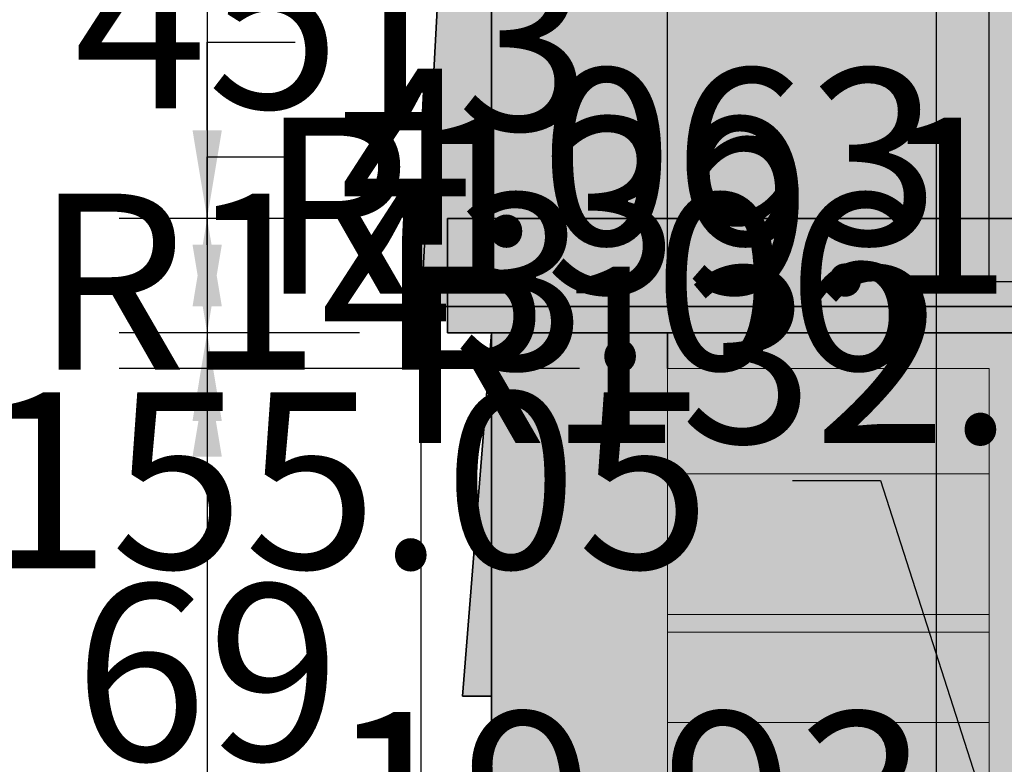
# Model space of a CAD drawing. Units: millimetres. Extents: x 130 to 1021, y 147 to 699.
# Tile 17 of 40: x 254 to 366, y 525 to 610. Entities that reach past the tile are written whole.
import ezdxf

# ---------------------------------------------------------------- set-up
doc = ezdxf.new("R2010")
doc.units = ezdxf.units.MM
doc.header["$MEASUREMENT"] = 0
for name, color, linetype, lineweight in [('A-ANNO-DIMS', 2, 'Continuous', 18), ('A-ELEV', 7, 'Continuous', 35), ('A-ELEV-PATT', 9, 'Continuous', 13), ('A-GLAZ', 4, 'Continuous', 18)]:
    doc.layers.add(name, color=color, linetype=linetype, lineweight=lineweight)
doc.styles.get("Standard").update_dxf_attribs({"font": 'arial.ttf'})
doc.dimstyles.get("Standard").update_dxf_attribs({"dimtxt": 20, "dimasz": 10, "dimexe": 10, "dimexo": 10, "dimgap": 5, "dimtad": 0, "dimtih": 1, "dimtoh": 1, "dimdec": 0, "dimzin": 0, "dimdsep": 46, "dimtxsty": 'Standard', "dimcen": 5, "dimadec": 0, "dimazin": 0, "dimtfac": 1, "dimtdec": 0, "dimtofl": 0, "dimtmove": 0, "dimatfit": 3, "dimfxl": 1, "dimtolj": 1, "dimtzin": 0, "dimarcsym": 0})

# ---------------------------------------------------------------- blocks, each defined once
blk = doc.blocks.new('*D11')
at = {"layer": 'A-ANNO-DIMS', "color": 0, "lineweight": -2, "transparency": 16777216}
for p, q in [((737.37, 648.7), (737.37, 149.74)), ((299.37, 566.95), (299.37, 149.74)), ((309.37, 159.74), (490.86, 159.74)), ((727.37, 159.74), (545.89, 159.74))]:
    blk.add_line(p, q, dxfattribs=at)
at = {"layer": 'A-ANNO-DIMS', "color": 0, "transparency": 16777216}
for points in [[(309.37, 161.41), (309.37, 158.07), (299.37, 159.74)], [(727.37, 161.41), (727.37, 158.07), (737.37, 159.74)]]:
    blk.add_solid(points, dxfattribs=at)
at = {"layer": 'Defpoints', "color": 0, "transparency": 16777216}
for p in [(737.37, 658.7), (299.37, 576.95), (737.37, 159.74)]:
    blk.add_point(p, dxfattribs=at)
at = {"layer": 'A-ANNO-DIMS', "color": 0, "transparency": 16777216, "insert": (518.37, 159.74), "char_height": 20, "attachment_point": 5}
blk.add_mtext('\\A1;438', dxfattribs=at)
blk = doc.blocks.new('*D12')
at = {"layer": 'A-ANNO-DIMS', "color": 0, "lineweight": -2, "transparency": 16777216}
for p, q in [((477.37, 661.95), (265.07, 661.95)), ((275.07, 651.95), (275.07, 438.2)), ((275.07, 194.04), (275.07, 407.78)), ((357.16, 184.04), (265.07, 184.04))]:
    blk.add_line(p, q, dxfattribs=at)
at = {"layer": 'A-ANNO-DIMS', "color": 0, "transparency": 16777216}
for points in [[(273.41, 651.95), (276.74, 651.95), (275.07, 661.95)], [(273.41, 194.04), (276.74, 194.04), (275.07, 184.04)]]:
    blk.add_solid(points, dxfattribs=at)
at = {"layer": 'Defpoints', "color": 0, "transparency": 16777216}
for p in [(275.07, 661.95), (487.37, 661.95), (367.16, 184.04)]:
    blk.add_point(p, dxfattribs=at)
at = {"layer": 'A-ANNO-DIMS', "color": 0, "transparency": 16777216, "insert": (275.07, 422.99), "char_height": 20, "attachment_point": 5}
blk.add_mtext('\\A1;477.9', dxfattribs=at)
blk = doc.blocks.new('*D14')
at = {"layer": 'A-ANNO-DIMS', "color": 0, "lineweight": -2, "transparency": 16777216}
for p, q in [((307.37, 641.95), (307.37, 696.25)), ((327.37, 579.88), (327.37, 696.25)), ((297.37, 686.25), (287.37, 686.25)), ((337.37, 686.25), (347.37, 686.25))]:
    blk.add_line(p, q, dxfattribs=at)
at = {"layer": 'A-ANNO-DIMS', "color": 0, "transparency": 16777216}
for points in [[(297.37, 687.91), (297.37, 684.58), (307.37, 686.25)], [(337.37, 687.91), (337.37, 684.58), (327.37, 686.25)]]:
    blk.add_solid(points, dxfattribs=at)
at = {"layer": 'Defpoints', "color": 0, "transparency": 16777216}
for p in [(327.37, 686.25), (307.37, 631.95), (327.37, 569.88)]:
    blk.add_point(p, dxfattribs=at)
at = {"layer": 'A-ANNO-DIMS', "color": 0, "transparency": 16777216, "insert": (366.83, 686.25), "char_height": 20, "attachment_point": 5}
blk.add_mtext('\\A1;20', dxfattribs=at)
blk = doc.blocks.new('*D15')
at = {"layer": 'A-ANNO-DIMS', "color": 0, "lineweight": -2, "transparency": 16777216}
for p, q in [((327.37, 579.88), (327.37, 696.25)), ((357.94, 411.95), (357.94, 696.25)), ((337.37, 686.25), (347.94, 686.25)), ((357.94, 686.25), (367.94, 686.25))]:
    blk.add_line(p, q, dxfattribs=at)
at = {"layer": 'A-ANNO-DIMS', "color": 0, "transparency": 16777216}
for points in [[(337.37, 687.91), (337.37, 684.58), (327.37, 686.25)], [(347.94, 687.91), (347.94, 684.58), (357.94, 686.25)]]:
    blk.add_solid(points, dxfattribs=at)
at = {"layer": 'Defpoints', "color": 0, "transparency": 16777216}
for p in [(357.94, 686.25), (327.37, 569.88), (357.94, 401.95)]:
    blk.add_point(p, dxfattribs=at)
at = {"layer": 'A-ANNO-DIMS', "color": 0, "transparency": 16777216, "insert": (406.68, 686.25), "char_height": 20, "attachment_point": 5}
blk.add_mtext('\\A1;30.57', dxfattribs=at)
blk = doc.blocks.new('*D16')
at = {"layer": 'A-ANNO-DIMS', "color": 0, "lineweight": -2, "transparency": 16777216}
for p, q in [((357.94, 411.95), (357.94, 696.25)), ((363.92, 579.88), (363.92, 696.25)), ((347.94, 686.25), (337.94, 686.25)), ((373.92, 686.25), (383.92, 686.25))]:
    blk.add_line(p, q, dxfattribs=at)
at = {"layer": 'A-ANNO-DIMS', "color": 0, "transparency": 16777216}
for points in [[(347.94, 687.91), (347.94, 684.58), (357.94, 686.25)], [(373.92, 687.91), (373.92, 684.58), (363.92, 686.25)]]:
    blk.add_solid(points, dxfattribs=at)
at = {"layer": 'Defpoints', "color": 0, "transparency": 16777216}
for p in [(363.92, 686.25), (363.92, 569.88), (357.94, 401.95)]:
    blk.add_point(p, dxfattribs=at)
at = {"layer": 'A-ANNO-DIMS', "color": 0, "transparency": 16777216, "insert": (420.74, 686.25), "char_height": 20, "attachment_point": 5}
blk.add_mtext('\\A1;5.981', dxfattribs=at)
blk = doc.blocks.new('*D17')
at = {"layer": 'A-ANNO-DIMS', "color": 0, "lineweight": -2, "transparency": 16777216}
for p, q in [((363.92, 579.88), (363.92, 696.25)), ((375.85, 490.22), (375.85, 696.25)), ((353.92, 686.25), (343.92, 686.25)), ((385.85, 686.25), (395.85, 686.25))]:
    blk.add_line(p, q, dxfattribs=at)
at = {"layer": 'A-ANNO-DIMS', "color": 0, "transparency": 16777216}
for points in [[(353.92, 687.91), (353.92, 684.58), (363.92, 686.25)], [(385.85, 687.91), (385.85, 684.58), (375.85, 686.25)]]:
    blk.add_solid(points, dxfattribs=at)
at = {"layer": 'Defpoints', "color": 0, "transparency": 16777216}
for p in [(375.85, 686.25), (363.92, 569.88), (375.85, 480.22)]:
    blk.add_point(p, dxfattribs=at)
at = {"layer": 'A-ANNO-DIMS', "color": 0, "transparency": 16777216, "insert": (441.44, 686.25), "char_height": 20, "attachment_point": 5}
blk.add_mtext('\\A1;11.928', dxfattribs=at)
blk = doc.blocks.new('*D18')
at = {"layer": 'A-ANNO-DIMS', "color": 0, "lineweight": -2, "transparency": 16777216}
for p, q in [((375.85, 490.22), (375.85, 696.25)), ((382.37, 388.95), (382.37, 696.25)), ((365.85, 686.25), (355.85, 686.25)), ((392.37, 686.25), (402.37, 686.25))]:
    blk.add_line(p, q, dxfattribs=at)
at = {"layer": 'A-ANNO-DIMS', "color": 0, "transparency": 16777216}
for points in [[(365.85, 687.91), (365.85, 684.58), (375.85, 686.25)], [(392.37, 687.91), (392.37, 684.58), (382.37, 686.25)]]:
    blk.add_solid(points, dxfattribs=at)
at = {"layer": 'Defpoints', "color": 0, "transparency": 16777216}
for p in [(382.37, 686.25), (375.85, 480.22), (382.37, 378.95)]:
    blk.add_point(p, dxfattribs=at)
at = {"layer": 'A-ANNO-DIMS', "color": 0, "transparency": 16777216, "insert": (441.13, 686.25), "char_height": 20, "attachment_point": 5}
blk.add_mtext('\\A1;6.524', dxfattribs=at)
blk = doc.blocks.new('*D43')
at = {"layer": 'A-ANNO-DIMS', "color": 0, "lineweight": -2, "transparency": 16777216}
for p, q in [((275.07, 510.88), (275.07, 520.88)), ((275.07, 520.88), (285.07, 520.88)), ((404.65, 500.88), (265.07, 500.88)), ((317.37, 480.95), (265.07, 480.95)), ((275.07, 470.95), (275.07, 460.95))]:
    blk.add_line(p, q, dxfattribs=at)
at = {"layer": 'A-ANNO-DIMS', "color": 0, "transparency": 16777216}
for points in [[(273.41, 510.88), (276.74, 510.88), (275.07, 500.88)], [(273.41, 470.95), (276.74, 470.95), (275.07, 480.95)]]:
    blk.add_solid(points, dxfattribs=at)
at = {"layer": 'Defpoints', "color": 0, "transparency": 16777216}
for p in [(275.07, 500.88), (414.65, 500.88), (327.37, 480.95)]:
    blk.add_point(p, dxfattribs=at)
at = {"layer": 'A-ANNO-DIMS', "color": 0, "transparency": 16777216, "insert": (322.88, 520.88), "char_height": 20, "attachment_point": 5}
blk.add_mtext('\\A1;19.93', dxfattribs=at)
blk = doc.blocks.new('*D44')
at = {"layer": 'A-ANNO-DIMS', "color": 0, "lineweight": -2, "transparency": 16777216}
for p, q in [((317.37, 569.88), (265.07, 569.88)), ((275.07, 559.88), (275.07, 550.59)), ((275.07, 510.88), (275.07, 520.17)), ((404.65, 500.88), (265.07, 500.88))]:
    blk.add_line(p, q, dxfattribs=at)
at = {"layer": 'A-ANNO-DIMS', "color": 0, "transparency": 16777216}
for points in [[(273.41, 559.88), (276.74, 559.88), (275.07, 569.88)], [(273.41, 510.88), (276.74, 510.88), (275.07, 500.88)]]:
    blk.add_solid(points, dxfattribs=at)
at = {"layer": 'Defpoints', "color": 0, "transparency": 16777216}
for p in [(275.07, 569.88), (327.37, 569.88), (414.65, 500.88)]:
    blk.add_point(p, dxfattribs=at)
at = {"layer": 'A-ANNO-DIMS', "color": 0, "transparency": 16777216, "insert": (275.07, 535.38), "char_height": 20, "attachment_point": 5}
blk.add_mtext('\\A1;69', dxfattribs=at)
blk = doc.blocks.new('*D45')
at = {"layer": 'A-ANNO-DIMS', "color": 0, "lineweight": -2, "transparency": 16777216}
for p, q in [((275.07, 583.95), (275.07, 593.95)), ((275.07, 593.95), (285.07, 593.95)), ((292.37, 573.95), (265.07, 573.95)), ((317.37, 569.88), (265.07, 569.88)), ((275.07, 559.88), (275.07, 549.88))]:
    blk.add_line(p, q, dxfattribs=at)
at = {"layer": 'A-ANNO-DIMS', "color": 0, "transparency": 16777216}
for points in [[(273.41, 583.95), (276.74, 583.95), (275.07, 573.95)], [(273.41, 559.88), (276.74, 559.88), (275.07, 569.88)]]:
    blk.add_solid(points, dxfattribs=at)
at = {"layer": 'Defpoints', "color": 0, "transparency": 16777216}
for p in [(275.07, 573.95), (302.37, 573.95), (327.37, 569.88)]:
    blk.add_point(p, dxfattribs=at)
at = {"layer": 'A-ANNO-DIMS', "color": 0, "transparency": 16777216, "insert": (324.22, 593.95), "char_height": 20, "attachment_point": 5}
blk.add_mtext('\\A1;4.063', dxfattribs=at)
blk = doc.blocks.new('*D46')
at = {"layer": 'A-ANNO-DIMS', "color": 0, "lineweight": -2, "transparency": 16777216}
for p, q in [((275.07, 596.95), (275.07, 606.95)), ((275.07, 606.95), (285.07, 606.95)), ((292.37, 586.95), (265.07, 586.95)), ((292.37, 573.95), (265.07, 573.95)), ((275.07, 563.95), (275.07, 553.95))]:
    blk.add_line(p, q, dxfattribs=at)
at = {"layer": 'A-ANNO-DIMS', "color": 0, "transparency": 16777216}
for points in [[(273.41, 596.95), (276.74, 596.95), (275.07, 586.95)], [(273.41, 563.95), (276.74, 563.95), (275.07, 573.95)]]:
    blk.add_solid(points, dxfattribs=at)
at = {"layer": 'Defpoints', "color": 0, "transparency": 16777216}
for p in [(275.07, 586.95), (302.37, 586.95), (302.37, 573.95)]:
    blk.add_point(p, dxfattribs=at)
at = {"layer": 'A-ANNO-DIMS', "color": 0, "transparency": 16777216, "insert": (303.46, 606.95), "char_height": 20, "attachment_point": 5}
blk.add_mtext('\\A1;13', dxfattribs=at)
blk = doc.blocks.new('*D47')
at = {"layer": 'A-ANNO-DIMS', "color": 0, "lineweight": -2, "transparency": 16777216}
for p, q in [((275.07, 641.95), (275.07, 651.95)), ((292.37, 631.95), (265.07, 631.95)), ((292.37, 586.95), (265.07, 586.95)), ((275.07, 576.95), (275.07, 566.95))]:
    blk.add_line(p, q, dxfattribs=at)
at = {"layer": 'A-ANNO-DIMS', "color": 0, "transparency": 16777216}
for points in [[(273.41, 641.95), (276.74, 641.95), (275.07, 631.95)], [(273.41, 576.95), (276.74, 576.95), (275.07, 586.95)]]:
    blk.add_solid(points, dxfattribs=at)
at = {"layer": 'Defpoints', "color": 0, "transparency": 16777216}
for p in [(275.07, 631.95), (302.37, 631.95), (302.37, 586.95)]:
    blk.add_point(p, dxfattribs=at)
at = {"layer": 'A-ANNO-DIMS', "color": 0, "transparency": 16777216, "insert": (275.07, 609.45), "char_height": 20, "attachment_point": 5}
blk.add_mtext('\\A1;45', dxfattribs=at)
blk = doc.blocks.new('*D66')
at = {"layer": 'A-ANNO-DIMS', "color": 0, "lineweight": -2, "transparency": 16777216}
for p, q in [((341.58, 557.19), (351.58, 557.19)), ((351.58, 557.19), (376.95, 478.14)), ((427.37, 315.98), (427.37, 325.98)), ((422.37, 320.98), (432.37, 320.98))]:
    blk.add_line(p, q, dxfattribs=at)
at = {"layer": 'A-ANNO-DIMS', "color": 0, "transparency": 16777216}
blk.add_solid([(378.53, 478.64), (375.36, 477.63), (380, 468.61)], dxfattribs=at)
at = {"layer": 'Defpoints', "color": 0, "transparency": 16777216}
for p in [(380, 468.61), (427.37, 320.98)]:
    blk.add_point(p, dxfattribs=at)
at = {"layer": 'A-ANNO-DIMS', "color": 0, "transparency": 16777216, "insert": (263.53, 557.19), "char_height": 20, "attachment_point": 5}
blk.add_mtext('\\A1;4X R155.05', dxfattribs=at)
blk = doc.blocks.new('*D68')
at = {"layer": 'A-ANNO-DIMS', "color": 0, "lineweight": -2, "transparency": 16777216}
for p, q in [((361.84, 579.76), (371.84, 579.76)), ((371.84, 579.76), (392.17, 506.69)), ((433.19, 354.23), (433.19, 364.23)), ((428.19, 359.23), (438.19, 359.23))]:
    blk.add_line(p, q, dxfattribs=at)
at = {"layer": 'A-ANNO-DIMS', "color": 0, "transparency": 16777216}
blk.add_solid([(393.77, 507.14), (390.56, 506.25), (394.85, 497.06)], dxfattribs=at)
at = {"layer": 'Defpoints', "color": 0, "transparency": 16777216}
for p in [(394.85, 497.06), (433.19, 359.23)]:
    blk.add_point(p, dxfattribs=at)
at = {"layer": 'A-ANNO-DIMS', "color": 0, "transparency": 16777216, "insert": (305.76, 579.76), "char_height": 20, "attachment_point": 5}
blk.add_mtext('\\A1;R143.06', dxfattribs=at)
blk = doc.blocks.new('*D70')
at = {"layer": 'A-ANNO-DIMS', "color": 0, "lineweight": -2, "transparency": 16777216}
for p, q in [((370.14, 588.4), (380.14, 588.4)), ((380.14, 588.4), (397.47, 517.01)), ((432.65, 367.11), (432.65, 377.11)), ((427.65, 372.11), (437.65, 372.11))]:
    blk.add_line(p, q, dxfattribs=at)
at = {"layer": 'A-ANNO-DIMS', "color": 0, "transparency": 16777216}
blk.add_solid([(399.09, 517.4), (395.85, 516.62), (399.83, 507.29)], dxfattribs=at)
at = {"layer": 'Defpoints', "color": 0, "transparency": 16777216}
for p in [(399.83, 507.29), (432.65, 372.11)]:
    blk.add_point(p, dxfattribs=at)
at = {"layer": 'A-ANNO-DIMS', "color": 0, "transparency": 16777216, "insert": (323.76, 588.4), "char_height": 20, "attachment_point": 5}
blk.add_mtext('\\A1;R139.1', dxfattribs=at)
blk = doc.blocks.new('*D73')
at = {"layer": 'A-ANNO-DIMS', "color": 0, "lineweight": -2, "transparency": 16777216}
for p, q in [((402.68, 571.45), (412.68, 571.45)), ((412.68, 571.45), (419.05, 502.17)), ((432.11, 355.14), (432.11, 365.14)), ((427.11, 360.14), (437.11, 360.14))]:
    blk.add_line(p, q, dxfattribs=at)
at = {"layer": 'A-ANNO-DIMS', "color": 0, "transparency": 16777216}
blk.add_solid([(420.71, 502.32), (417.39, 502.01), (419.97, 492.21)], dxfattribs=at)
at = {"layer": 'Defpoints', "color": 0, "transparency": 16777216}
for p in [(419.97, 492.21), (432.11, 360.14)]:
    blk.add_point(p, dxfattribs=at)
at = {"layer": 'A-ANNO-DIMS', "color": 0, "transparency": 16777216, "insert": (346.7, 571.45), "char_height": 20, "attachment_point": 5}
blk.add_mtext('\\A1;R132.62', dxfattribs=at)

msp = doc.modelspace()

# ---------------------------------------------------------------- hatches: boundary and pattern name
at = {"layer": 'A-ELEV-PATT'}
h = msp.add_hatch(color=256, dxfattribs=at)
h.dxf.hatch_style = 1
h.paths.add_polyline_path([(737.3738, 658.6988, 0.01359606), (632.4019, 661.9473), (607.3738, 661.9473), (487.3738, 661.9473), (487.3738, 649.9473), (607.3738, 649.9473), (632.3794, 649.9473, -0.01368411), (737.3738, 646.6784)])
h.paths.add_polyline_path([(732.3738, 643.9599, 0.01305286), (632.3738, 646.9473), (607.3738, 646.9473), (487.3738, 646.9473), (487.3738, 596.9473), (632.3738, 596.9473, -0.01305286), (732.3738, 593.9599)])
h.paths.add_polyline_path([(737.3738, 593.6732, 0.01370629), (632.3738, 596.9473), (487.3738, 596.9473), (487.3738, 586.9473), (632.355, 586.9473, -0.01378075), (737.3738, 583.6559)])
h.paths.add_polyline_path([(447.3738, 646.9473), (307.3738, 646.9473), (302.3738, 646.9473), (302.3738, 634.9473), (447.3738, 634.9473)])
h.paths.add_polyline_path([(447.3738, 631.9473), (307.3738, 631.9473), (307.3738, 586.9473), (447.3738, 586.9473)])
h.paths.add_polyline_path([(447.3738, 586.9473), (307.3738, 586.9473), (302.3738, 586.9473), (302.3738, 576.9473), (447.3738, 576.9473)])
h.paths.add_polyline_path([(447.3738, 573.9473), (367.3738, 573.9473), (367.3738, 539.9473), (447.3738, 539.9473)])
h.paths.add_polyline_path([(447.3738, 537.9473), (367.3738, 537.9473), (367.3738, 507.9473), (400.392, 507.4253, -0.00172798), (401.3281, 507.6451, -0.52200255), (425.6117, 511.0391, -0.03918489), (447.3738, 510.4359), (447.3738, 510.7883)])
h.paths.add_polyline_path([(394.7238, 505.9473), (367.3738, 505.9473), (367.3738, 476.9473, -0.0146512), (375.8501, 480.2159), (376.1506, 499.2266, -0.03554194)])
h.paths.add_polyline_path([(632.3738, 583.9473), (552.3738, 583.9473), (552.3738, 550.9473), (632.3738, 550.9473)])
h.paths.add_polyline_path([(632.3738, 548.9473), (552.3738, 548.9473), (552.3738, 515.9473), (632.3738, 515.9473)])
h.paths.add_polyline_path([(632.3738, 513.9473), (552.3738, 513.9473), (552.3738, 476.9473), (632.3738, 476.9473)])
h.paths.add_polyline_path([(737.3738, 473.6903, 0.01363261), (632.3926, 476.9473), (552.3738, 476.9473), (487.3738, 476.9473), (487.3738, 466.9473), (632.3738, 466.9473, -0.01370629), (737.3738, 463.6732)])
h.paths.add_polyline_path([(732.3738, 460.9552, 0.01307409), (632.3681, 463.9473), (487.3738, 463.9473), (487.3738, 407.735, -0.00322862), (489.3544, 406.9473), (632.3926, 406.9473, -0.01298259), (732.3738, 403.9755)])
h.paths.add_polyline_path([(487.3738, 463.9473, 0.20132998), (367.3738, 463.9473), (367.3738, 407.735, -0.18820307), (487.3738, 407.735)])
h.paths.add_polyline_path([(367.3738, 476.9473), (367.3738, 466.9473, -0.20133085), (487.3738, 466.9473), (487.3738, 476.9473, 0.20132998)])
h.paths.add_polyline_path([(367.3738, 463.9473), (307.3738, 463.9473), (307.3738, 401.9473), (357.9413, 401.9473), (367.3738, 407.735)])
h.paths.add_polyline_path([(367.3738, 476.9473), (302.3738, 476.9473), (302.3738, 466.9473), (367.3738, 466.9473)])
h.paths.add_polyline_path([(632.8184, 366.9453), (552.3738, 366.9453), (552.3738, 393.9473), (632.8184, 393.9473)])
h.paths.add_polyline_path([(632.8184, 357.2114), (632.8184, 363.9453), (552.3738, 363.9453), (552.3738, 357.2114), (552.3738, 336.9453), (632.8184, 336.9453)])
h.paths.add_polyline_path([(632.8184, 333.9453), (552.3738, 333.9453), (552.3738, 306.9453), (632.8184, 306.9453)])
h.paths.add_polyline_path([(632.8184, 303.9453), (552.3738, 303.9453), (552.3738, 273.9473), (632.355, 273.9473, 0.00006077), (632.8184, 273.9491)])
h.paths.add_polyline_path([(737.3738, 403.6903, 0.01363261), (632.3926, 406.9473), (489.3544, 406.9473, 0.19154808), (367.3738, 407.735), (367.3738, 396.9473, -0.20133085), (487.3738, 396.9473), (632.3738, 396.9473, -0.01370629), (737.3738, 393.6732)])
h.paths.add_polyline_path([(357.9413, 401.9473), (307.3738, 401.9473), (307.3738, 391.9473), (357.9413, 391.9473)])
h.paths.add_polyline_path([(357.9413, 357.2114), (357.9413, 388.9473), (307.3738, 388.9473), (307.3738, 357.2114), (307.3738, 273.9473), (357.9413, 273.9473)])
h.paths.add_polyline_path([(732.3738, 263.93, -0.0130317), (632.3794, 260.9473), (466.7667, 260.9473), (466.7667, 240.9473), (469.8406, 236.978), (469.8406, 221.978), (472.9145, 218.0087), (472.9145, 213.9473), (607.3738, 213.9473), (732.3738, 213.9473)])
h.paths.add_polyline_path([(732.3738, 290.889), (722.479, 290.889), (722.479, 301.889), (732.3738, 301.889), (732.3738, 305.889), (722.479, 305.889), (722.479, 316.889), (732.3738, 316.889), (732.3738, 320.889), (722.479, 320.889), (722.479, 331.889), (732.3738, 331.889), (732.3738, 335.889), (722.479, 335.889), (722.479, 346.889), (732.3738, 346.889), (732.3738, 350.889), (722.479, 350.889), (722.479, 361.889), (732.3738, 361.889), (732.3738, 365.889), (722.479, 365.889), (722.479, 376.889), (732.3738, 376.889), (732.3738, 380.889), (722.479, 380.889), (722.479, 391.4848, 0.00052326), (718.479, 391.6843), (718.479, 380.889), (707.479, 380.889), (707.479, 392.1896, 0.00052307), (703.479, 392.3576), (703.479, 380.889), (692.479, 380.889), (692.479, 392.7765, 0.00052292), (688.479, 392.9131), (688.479, 380.889), (677.479, 380.889), (677.479, 393.2456, 0.00052279), (673.479, 393.3508), (673.479, 380.889), (662.479, 380.889), (662.479, 393.597, 0.0005227), (658.479, 393.6709), (658.479, 380.889), (647.479, 380.889), (647.479, 393.8308, 0.00052264), (643.479, 393.8732), (643.479, 380.889), (632.8184, 380.889), (632.8184, 376.889), (643.479, 376.889), (643.479, 365.889), (632.8184, 365.889), (632.8184, 361.889), (643.479, 361.889), (643.479, 350.889), (632.8184, 350.889), (632.8184, 346.889), (643.479, 346.889), (643.479, 335.889), (632.8184, 335.889), (632.8184, 331.889), (643.479, 331.889), (643.479, 320.889), (632.8184, 320.889), (632.8184, 316.889), (643.479, 316.889), (643.479, 305.889), (632.8184, 305.889), (632.8184, 301.889), (643.479, 301.889), (643.479, 290.889), (632.8184, 290.889), (632.8184, 286.889), (643.479, 286.889), (643.479, 274.0217, 0.00052456), (647.479, 274.0643), (647.479, 286.889), (658.479, 286.889), (658.479, 274.2248, 0.00052462), (662.479, 274.2989), (662.479, 286.889), (673.479, 286.889), (673.479, 274.546, 0.00052471), (677.479, 274.6516), (677.479, 286.889), (688.479, 286.889), (688.479, 274.9853, 0.00052484), (692.479, 275.1224), (692.479, 286.889), (703.479, 286.889), (703.479, 275.5429, 0.000525), (707.479, 275.7115), (707.479, 286.889), (718.479, 286.889), (718.479, 276.2187, 0.00052519), (722.479, 276.4189), (722.479, 286.889), (732.3738, 286.889)])
h.paths.add_polyline_path([(718.479, 290.889), (707.479, 290.889), (707.479, 301.889), (718.479, 301.889)], flags=16)
h.paths.add_polyline_path([(703.479, 290.889), (692.479, 290.889), (692.479, 301.889), (703.479, 301.889)], flags=16)
h.paths.add_polyline_path([(718.479, 305.889), (707.479, 305.889), (707.479, 316.889), (718.479, 316.889)], flags=16)
h.paths.add_polyline_path([(703.479, 305.889), (692.479, 305.889), (692.479, 316.889), (703.479, 316.889)], flags=16)
h.paths.add_polyline_path([(688.479, 290.889), (677.479, 290.889), (677.479, 301.889), (688.479, 301.889)], flags=16)
h.paths.add_polyline_path([(718.479, 320.889), (707.479, 320.889), (707.479, 331.889), (718.479, 331.889)], flags=16)
h.paths.add_polyline_path([(688.479, 305.889), (677.479, 305.889), (677.479, 316.889), (688.479, 316.889)], flags=16)
h.paths.add_polyline_path([(703.479, 320.889), (692.479, 320.889), (692.479, 331.889), (703.479, 331.889)], flags=16)
h.paths.add_polyline_path([(688.479, 320.889), (677.479, 320.889), (677.479, 331.889), (688.479, 331.889)], flags=16)
h.paths.add_polyline_path([(673.479, 290.889), (662.479, 290.889), (662.479, 301.889), (673.479, 301.889)], flags=16)
h.paths.add_polyline_path([(718.479, 335.889), (707.479, 335.889), (707.479, 346.889), (718.479, 346.889)], flags=16)
h.paths.add_polyline_path([(673.479, 305.889), (662.479, 305.889), (662.479, 316.889), (673.479, 316.889)], flags=16)
h.paths.add_polyline_path([(703.479, 335.889), (692.479, 335.889), (692.479, 346.889), (703.479, 346.889)], flags=16)
h.paths.add_polyline_path([(673.479, 320.889), (662.479, 320.889), (662.479, 331.889), (673.479, 331.889)], flags=16)
h.paths.add_polyline_path([(688.479, 335.889), (677.479, 335.889), (677.479, 346.889), (688.479, 346.889)], flags=16)
h.paths.add_polyline_path([(658.479, 290.889), (647.479, 290.889), (647.479, 301.889), (658.479, 301.889)], flags=16)
h.paths.add_polyline_path([(718.479, 350.889), (707.479, 350.889), (707.479, 361.889), (718.479, 361.889)], flags=16)
h.paths.add_polyline_path([(658.479, 305.889), (647.479, 305.889), (647.479, 316.889), (658.479, 316.889)], flags=16)
h.paths.add_polyline_path([(703.479, 350.889), (692.479, 350.889), (692.479, 361.889), (703.479, 361.889)], flags=16)
h.paths.add_polyline_path([(673.479, 335.889), (662.479, 335.889), (662.479, 346.889), (673.479, 346.889)], flags=16)
h.paths.add_polyline_path([(658.479, 320.889), (647.479, 320.889), (647.479, 331.889), (658.479, 331.889)], flags=16)
h.paths.add_polyline_path([(688.479, 350.889), (677.479, 350.889), (677.479, 361.889), (688.479, 361.889)], flags=16)
h.paths.add_polyline_path([(718.479, 365.889), (707.479, 365.889), (707.479, 376.889), (718.479, 376.889)], flags=16)
h.paths.add_polyline_path([(658.479, 335.889), (647.479, 335.889), (647.479, 346.889), (658.479, 346.889)], flags=16)
h.paths.add_polyline_path([(673.479, 350.889), (662.479, 350.889), (662.479, 361.889), (673.479, 361.889)], flags=16)
h.paths.add_polyline_path([(703.479, 365.889), (692.479, 365.889), (692.479, 376.889), (703.479, 376.889)], flags=16)
h.paths.add_polyline_path([(688.479, 365.889), (677.479, 365.889), (677.479, 376.889), (688.479, 376.889)], flags=16)
h.paths.add_polyline_path([(658.479, 350.889), (647.479, 350.889), (647.479, 361.889), (658.479, 361.889)], flags=16)
h.paths.add_polyline_path([(673.479, 365.889), (662.479, 365.889), (662.479, 376.889), (673.479, 376.889)], flags=16)
h.paths.add_polyline_path([(658.479, 365.889), (647.479, 365.889), (647.479, 376.889), (658.479, 376.889)], flags=16)
h.paths.add_polyline_path([(732.3738, 503.9786), (722.3392, 503.9786), (722.3392, 514.9786), (732.3738, 514.9786), (732.3738, 518.9786), (722.3392, 518.9786), (722.3392, 529.9786), (732.3738, 529.9786), (732.3738, 533.9786), (722.3392, 533.9786), (722.3392, 544.9786), (732.3738, 544.9786), (732.3738, 546.9473), (732.3738, 548.9786), (722.3392, 548.9786), (722.3392, 559.9786), (732.3738, 559.9786), (732.3738, 563.9786), (722.3392, 563.9786), (722.3392, 574.9786), (732.3738, 574.9786), (732.3738, 578.9786), (722.3392, 578.9786), (722.3392, 581.4789, 0.00052601), (718.3392, 581.6791), (718.3392, 578.9786), (707.3392, 578.9786), (707.3392, 582.1863, 0.00052582), (703.3392, 582.355), (703.3392, 578.9786), (692.3392, 578.9786), (692.3392, 582.7752, 0.00052566), (688.3392, 582.9123), (688.3392, 578.9786), (677.3392, 578.9786), (677.3392, 583.2457, 0.00052554), (673.3392, 583.3512), (673.3392, 578.9786), (662.3392, 578.9786), (662.3392, 583.5978, 0.00052545), (658.3392, 583.6718), (658.3392, 578.9786), (647.3392, 578.9786), (647.3392, 583.8317, 0.00052539), (643.3392, 583.8741), (643.3392, 578.9786), (632.3738, 578.9786), (632.3738, 574.9786), (643.3392, 574.9786), (643.3392, 563.9786), (632.3738, 563.9786), (632.3738, 559.9786), (643.3392, 559.9786), (643.3392, 548.9786), (632.3738, 548.9786), (632.3738, 544.9786), (643.3392, 544.9786), (643.3392, 533.9786), (632.3738, 533.9786), (632.3738, 529.9786), (643.3392, 529.9786), (643.3392, 518.9786), (632.3738, 518.9786), (632.3738, 515.9473), (632.3738, 514.9786), (643.3392, 514.9786), (643.3392, 503.9786), (632.3738, 503.9786), (632.3738, 499.9786), (643.3392, 499.9786), (643.3392, 488.9786), (632.3738, 488.9786), (632.3738, 484.9786), (643.3392, 484.9786), (643.3392, 476.8751, -0.00051911), (647.3392, 476.8332), (647.3392, 484.9786), (658.3392, 484.9786), (658.3392, 476.6752, -0.00051917), (662.3392, 476.6022), (662.3392, 484.9786), (673.3392, 484.9786), (673.3392, 476.3585, -0.00051926), (677.3392, 476.2543), (677.3392, 484.9786), (688.3392, 484.9786), (688.3392, 475.9248, -0.00051938), (692.3392, 475.7894), (692.3392, 484.9786), (703.3392, 484.9786), (703.3392, 475.3741, -0.00051953), (707.3392, 475.2075), (707.3392, 484.9786), (718.3392, 484.9786), (718.3392, 474.7064, -0.00051972), (722.3392, 474.5086), (722.3392, 484.9786), (732.3738, 484.9786), (732.3738, 488.9786), (722.3392, 488.9786), (722.3392, 499.9786), (732.3738, 499.9786)])
h.paths.add_polyline_path([(718.3392, 503.9786), (707.3392, 503.9786), (707.3392, 514.9786), (718.3392, 514.9786)], flags=16)
h.paths.add_polyline_path([(718.3392, 499.9786), (718.3392, 488.9786), (707.3392, 488.9786), (707.3392, 499.9786)], flags=16)
h.paths.add_polyline_path([(718.3392, 518.9786), (707.3392, 518.9786), (707.3392, 529.9786), (718.3392, 529.9786)], flags=16)
h.paths.add_polyline_path([(703.3392, 503.9786), (692.3392, 503.9786), (692.3392, 514.9786), (703.3392, 514.9786)], flags=16)
h.paths.add_polyline_path([(703.3392, 499.9786), (703.3392, 488.9786), (692.3392, 488.9786), (692.3392, 499.9786)], flags=16)
h.paths.add_polyline_path([(703.3392, 518.9786), (692.3392, 518.9786), (692.3392, 529.9786), (703.3392, 529.9786)], flags=16)
h.paths.add_polyline_path([(718.3392, 533.9786), (707.3392, 533.9786), (707.3392, 544.9786), (718.3392, 544.9786)], flags=16)
h.paths.add_polyline_path([(688.3392, 503.9786), (677.3392, 503.9786), (677.3392, 514.9786), (688.3392, 514.9786)], flags=16)
h.paths.add_polyline_path([(688.3392, 499.9786), (688.3392, 488.9786), (677.3392, 488.9786), (677.3392, 499.9786)], flags=16)
h.paths.add_polyline_path([(703.3392, 533.9786), (692.3392, 533.9786), (692.3392, 544.9786), (703.3392, 544.9786)], flags=16)
h.paths.add_polyline_path([(688.3392, 518.9786), (677.3392, 518.9786), (677.3392, 529.9786), (688.3392, 529.9786)], flags=16)
h.paths.add_polyline_path([(688.3392, 533.9786), (677.3392, 533.9786), (677.3392, 544.9786), (688.3392, 544.9786)], flags=16)
h.paths.add_polyline_path([(718.3392, 548.9786), (707.3392, 548.9786), (707.3392, 559.9786), (718.3392, 559.9786)], flags=16)
h.paths.add_polyline_path([(673.3392, 503.9786), (662.3392, 503.9786), (662.3392, 514.9786), (673.3392, 514.9786)], flags=16)
h.paths.add_polyline_path([(673.3392, 499.9786), (673.3392, 488.9786), (662.3392, 488.9786), (662.3392, 499.9786)], flags=16)
h.paths.add_polyline_path([(703.3392, 548.9786), (692.3392, 548.9786), (692.3392, 559.9786), (703.3392, 559.9786)], flags=16)
h.paths.add_polyline_path([(673.3392, 518.9786), (662.3392, 518.9786), (662.3392, 529.9786), (673.3392, 529.9786)], flags=16)
h.paths.add_polyline_path([(688.3392, 548.9786), (677.3392, 548.9786), (677.3392, 559.9786), (688.3392, 559.9786)], flags=16)
h.paths.add_polyline_path([(673.3392, 533.9786), (662.3392, 533.9786), (662.3392, 544.9786), (673.3392, 544.9786)], flags=16)
h.paths.add_polyline_path([(718.3392, 563.9786), (707.3392, 563.9786), (707.3392, 574.9786), (718.3392, 574.9786)], flags=16)
h.paths.add_polyline_path([(658.3392, 503.9786), (647.3392, 503.9786), (647.3392, 514.9786), (658.3392, 514.9786)], flags=16)
h.paths.add_polyline_path([(658.3392, 499.9786), (658.3392, 488.9786), (647.3392, 488.9786), (647.3392, 499.9786)], flags=16)
h.paths.add_polyline_path([(703.3392, 563.9786), (692.3392, 563.9786), (692.3392, 574.9786), (703.3392, 574.9786)], flags=16)
h.paths.add_polyline_path([(658.3392, 518.9786), (647.3392, 518.9786), (647.3392, 529.9786), (658.3392, 529.9786)], flags=16)
h.paths.add_polyline_path([(673.3392, 548.9786), (662.3392, 548.9786), (662.3392, 559.9786), (673.3392, 559.9786)], flags=16)
h.paths.add_polyline_path([(688.3392, 563.9786), (677.3392, 563.9786), (677.3392, 574.9786), (688.3392, 574.9786)], flags=16)
h.paths.add_polyline_path([(658.3392, 533.9786), (647.3392, 533.9786), (647.3392, 544.9786), (658.3392, 544.9786)], flags=16)
h.paths.add_polyline_path([(673.3392, 563.9786), (662.3392, 563.9786), (662.3392, 574.9786), (673.3392, 574.9786)], flags=16)
h.paths.add_polyline_path([(658.3392, 548.9786), (647.3392, 548.9786), (647.3392, 559.9786), (658.3392, 559.9786)], flags=16)
h.paths.add_polyline_path([(658.3392, 563.9786), (647.3392, 563.9786), (647.3392, 574.9786), (658.3392, 574.9786)], flags=16)
h = msp.add_hatch(color=256, dxfattribs=at)
h.paths.add_polyline_path([(299.3738, 576.9473), (302.3738, 576.9473), (302.3738, 586.9473), (307.3738, 586.9473), (307.3738, 631.9473), (302.3738, 631.9473)])
h.paths.add_polyline_path([(304.0806, 532.6995), (307.3738, 532.6995), (307.3738, 573.9473)])
h = msp.add_hatch(color=256, dxfattribs=at)
h.dxf.hatch_style = 1
h.paths.add_polyline_path([(447.3738, 576.9473), (302.3738, 576.9473), (302.3738, 573.9473), (447.3738, 573.9473)])
h.paths.add_polyline_path([(487.3738, 583.9473), (487.3738, 586.9473), (447.3738, 576.9473), (447.3738, 573.9473)])
h.paths.add_polyline_path([(632.355, 586.9473), (487.3738, 586.9473), (487.3738, 583.9473), (632.3738, 583.9473), (632.3738, 583.9472, -0.01380003), (737.3738, 580.6507), (737.3738, 583.6559, 0.01378075)])
h.paths.add_polyline_path([(367.3738, 466.9473), (302.3738, 466.9473), (302.3738, 463.9473), (367.3738, 463.9473)])
h.paths.add_polyline_path([(487.3738, 463.9473), (487.3738, 466.9473, 0.20133085), (367.3738, 466.9473), (367.3738, 463.9473, -0.20132998)])
h.paths.add_polyline_path([(632.3738, 466.9473), (487.3738, 466.9473), (487.3738, 463.9473), (632.3681, 463.9473, -0.01372855), (737.3738, 460.6681), (737.3738, 463.6732, 0.01370629)])
h.paths.add_polyline_path([(632.3738, 396.9473), (487.3738, 396.9473, 0.20133085), (367.3738, 396.9473), (367.3738, 393.9473, -0.20237172), (486.7667, 393.9473), (632.3681, 393.9473, -0.01372855), (737.3738, 390.6681), (737.3738, 393.6732, 0.01370629)])
h.paths.add_polyline_path([(357.9413, 391.9473), (307.3738, 391.9473), (307.3738, 388.9473), (357.9413, 388.9473)])
h.paths.add_polyline_path([(367.3738, 393.9473), (367.3738, 396.9473), (357.9413, 391.924), (357.9413, 388.9473), (358.058, 388.9473)])
h.paths.add_polyline_path([(737.3738, 264.2162), (737.3738, 267.2214, -0.01370629), (632.3738, 263.9473), (463.7667, 263.9473), (466.7667, 260.9473), (632.3794, 260.9473, 0.01368411)])
h.paths.add_polyline_path([(463.7667, 263.9473), (447.3738, 263.9473), (450.3738, 260.9473), (466.7667, 260.9473)])
h.paths.add_polyline_path([(447.3738, 263.9473), (432.3738, 263.9473), (432.3738, 260.9473), (450.3738, 260.9473)])
h.paths.add_polyline_path([(382.3738, 263.9473), (357.9413, 263.9473), (357.9413, 260.9473), (382.3738, 260.9473)])
h.paths.add_polyline_path([(357.9413, 263.9473), (307.3738, 263.9473), (307.3738, 260.9473), (357.9413, 260.9473)])
h = msp.add_hatch(color=256, dxfattribs=at)
h.paths.add_polyline_path([(327.3738, 569.884), (327.3738, 573.9473), (307.3738, 573.9473), (307.3738, 476.9473), (327.3738, 476.9473), (327.3738, 480.95)])
h.paths.add_polyline_path([(486.7667, 386.2639), (486.7667, 393.9473), (466.7667, 393.9473), (466.7667, 357.2114), (466.7667, 311.9335, 0.03427026), (486.7667, 308.4637)])
h.paths.add_polyline_path([(486.7667, 308.4637, -0.03427026), (466.7667, 311.9335), (466.7667, 273.9473), (486.7667, 273.9473)])
h.paths.add_polyline_path([(389.3738, 351.5473), (396.7693, 351.5473, -0.00702703), (393.8774, 354.5473), (389.3738, 354.5473), (389.3738, 359.5775, -0.01903024), (382.3738, 368.424), (382.3738, 249.5473), (432.3738, 249.5473), (432.3738, 325.067, -0.00576734), (429.3738, 326.709), (429.3738, 257.5473), (426.3738, 257.5473), (426.3738, 328.4428, -0.00592542), (423.3738, 330.272), (423.3738, 315.7473), (389.3738, 315.7473), (389.3738, 332.1473), (420.4552, 332.1473, -0.00895099), (416.0768, 335.1473), (389.3738, 335.1473)])
h.paths.add_polyline_path([(389.3738, 312.7473), (423.3738, 312.7473), (423.3738, 296.3473), (389.3738, 296.3473)], flags=16)
h.paths.add_polyline_path([(389.3738, 293.3473), (423.3738, 293.3473), (423.3738, 276.9473), (389.3738, 276.9473)], flags=16)
h.paths.add_polyline_path([(389.3738, 273.9473), (423.3738, 273.9473), (423.3738, 257.5473), (389.3738, 257.5473)], flags=16)
h.paths.add_polyline_path([(432.3738, 378.9473), (382.3738, 378.9473), (382.3738, 368.424, 0.01903024), (389.3738, 359.5775), (389.3738, 370.9473), (423.3738, 370.9473), (423.3738, 354.5473), (393.8774, 354.5473, 0.00702703), (396.7693, 351.5473), (423.3738, 351.5473), (423.3738, 335.1473), (416.0768, 335.1473, 0.00895099), (420.4552, 332.1473), (423.3738, 332.1473), (423.3738, 330.272, 0.00592542), (426.3738, 328.4428), (426.3738, 370.9473), (429.3738, 370.9473), (429.3738, 326.709, 0.00576734), (432.3738, 325.067)])
h.paths.add_polyline_path([(466.7667, 357.2114), (466.7667, 393.9473), (447.3738, 393.9473), (447.3738, 357.2114), (447.3738, 318.1243, 0.0063261), (450.8779, 316.785), (450.8779, 331.5915), (463.5608, 331.5915), (463.5608, 312.7571, 0.00558197), (466.7667, 311.9335)])
h.paths.add_polyline_path([(450.8779, 334.5915), (450.8779, 360.0915), (463.5608, 360.0915), (463.5608, 334.5915)], flags=16)
h.paths.add_polyline_path([(450.8779, 363.0915), (450.8779, 388.6449), (463.5608, 388.6449), (463.5608, 363.0915)], flags=16)
h.paths.add_polyline_path([(466.7667, 311.9335, -0.00558197), (463.5608, 312.7571), (463.5608, 306.0915), (450.8779, 306.0915), (450.8779, 316.785, -0.0063261), (447.3738, 318.1243), (447.3738, 273.9473), (466.7667, 273.9473)])
h.paths.add_polyline_path([(450.8779, 303.0915), (463.5608, 303.0915), (463.5608, 277.5915), (450.8779, 277.5915)], flags=16)
h.paths.add_polyline_path([(552.3738, 357.2114), (552.3738, 393.9473), (486.7667, 393.9473), (486.7667, 386.2639), (544.6354, 386.2639), (544.6354, 280.6619), (486.7667, 280.6619), (486.7667, 273.9473), (552.3738, 273.9473)])
h.paths.add_polyline_path([(487.3738, 583.9473), (472.3738, 580.1973), (472.3738, 507.0765), (472.3738, 505.4251, -0.00564525), (475.3738, 504.4942), (475.3738, 506.3543), (475.3738, 511.9473), (484.3738, 511.9473), (484.3738, 503.8134), (484.3738, 501.2439, -0.00583574), (487.3738, 500.0015)])
h.paths.add_polyline_path([(484.3738, 578.0434), (484.3738, 548.9473), (475.3738, 548.9473), (475.3738, 575.7934)], flags=16)
h.paths.add_polyline_path([(484.3738, 546.9473), (484.3738, 513.9473), (475.3738, 513.9473), (475.3738, 518.7148), (475.3738, 546.9473)], flags=16)
h = msp.add_hatch(color=256, dxfattribs=at)
h.dxf.hatch_style = 1
h.paths.add_polyline_path([(363.922, 569.884), (327.3738, 569.884), (327.3738, 557.9168), (363.922, 557.9168)])
h.paths.add_polyline_path([(547.7773, 577.3739), (502.3738, 577.3739), (502.3738, 566.2111), (547.7773, 566.2111)])
h.paths.add_polyline_path([(544.6354, 386.2639), (486.7667, 386.2639), (486.7667, 377.43), (544.6354, 377.43)])
h.paths.add_polyline_path([(496.0546, 377.43), (486.7667, 377.43), (486.7667, 370.4028)])
h.paths.add_polyline_path([(447.3738, 393.9473), (367.3738, 393.9473, 0.05004781), (382.3738, 368.424), (382.3738, 378.9473), (432.3738, 378.9473), (432.3738, 325.067, 0.02789446), (447.3738, 318.1243), (447.3738, 357.2114)])
h.paths.add_polyline_path([(463.5608, 388.6449), (450.8779, 388.6449), (450.8779, 363.0915), (463.5608, 363.0915)])
h.paths.add_polyline_path([(463.5608, 360.0915), (450.8779, 360.0915), (450.8779, 334.5915), (463.5608, 334.5915)])
h.paths.add_polyline_path([(463.5608, 331.5915), (450.8779, 331.5915), (450.8779, 316.785, 0.02245133), (463.5608, 312.7571)])
msp.add_hatch(color=256, dxfattribs=at).paths.add_polyline_path([(327.3738, 573.9473), (327.3738, 569.884), (363.922, 569.884), (363.922, 480.95), (327.3738, 480.95), (327.3738, 476.9473), (367.3738, 476.9473), (367.3738, 573.9473)])
h = msp.add_hatch(color=256, dxfattribs=at)
h.dxf.hatch_style = 1
h.paths.add_polyline_path([(363.922, 541.9473), (363.922, 557.9168), (327.3738, 557.9168), (327.3738, 541.9473)])
h.paths.add_polyline_path([(363.922, 529.7), (363.922, 539.9473), (327.3738, 539.9473), (327.3738, 529.7)])
h = msp.add_hatch(color=256, dxfattribs=at)
h.paths.add_polyline_path([(327.3738, 541.9473), (327.3738, 539.9473), (363.922, 539.9473), (363.922, 541.9473)])
h.paths.add_polyline_path([(327.3738, 509.9473), (327.3738, 507.9473), (363.922, 507.9473), (363.922, 509.9473)])
h = msp.add_hatch(color=256, dxfattribs=at)
h.dxf.hatch_style = 1
h.paths.add_polyline_path([(364.0891, 218.0087), (361.0152, 221.978), (361.0152, 236.978), (357.9413, 240.9473), (357.9413, 195.9473), (367.163, 184.0395), (367.163, 199.0395), (364.0891, 203.0087)])
h.paths.add_polyline_path([(502.3738, 537.2685), (502.3738, 513.9473), (547.7773, 513.9473), (547.7773, 537.2685)])
h.paths.add_polyline_path([(502.3738, 511.9473), (502.3738, 481.7432), (547.7773, 481.7432), (547.7773, 511.9473)])
h.paths.add_polyline_path([(327.3738, 529.7), (327.3738, 509.9473), (363.922, 509.9473), (363.922, 529.7)])
h.paths.add_polyline_path([(327.3738, 507.9473), (327.3738, 480.95), (363.922, 480.95), (363.922, 507.9473)])

# ---------------------------------------------------------------- linework, layer by layer
at = {"layer": 'A-ELEV'}
for p, q in [((299.3738, 576.9473), (302.3738, 631.9473)), ((307.3738, 631.9473), (307.3738, 586.9473)), ((447.3738, 586.9473), (302.3738, 586.9473)), ((302.3738, 586.9473), (302.3738, 573.9473)), ((302.3738, 576.9473), (299.3738, 576.9473)), ((447.3738, 576.9473), (302.3738, 576.9473)), ((447.3738, 573.9473), (302.3738, 573.9473)), ((304.0806, 532.6995), (307.3738, 573.9473)), ((307.3738, 573.9473), (307.3738, 476.9473)), ((327.3738, 569.884), (327.3738, 573.9473)), ((307.3738, 532.6995), (304.0806, 532.6995))]:
    msp.add_line(p, q, dxfattribs=at)
at = {"layer": 'A-GLAZ'}
for p, q in [((327.3738, 557.9168), (363.922, 557.9168)), ((363.922, 541.9473), (327.3738, 541.9473)), ((363.922, 539.9473), (327.3738, 539.9473)), ((327.3738, 529.7), (363.922, 529.7))]:
    msp.add_line(p, q, dxfattribs=at)
msp.add_lwpolyline([(363.922, 569.884), (327.3738, 569.884), (327.3738, 480.95), (363.922, 480.95)], close=True, dxfattribs=at)

# ---------------------------------------------------------------- dimensions: what is measured, and where the dimension line sits
at = {"layer": 'A-ANNO-DIMS'}
for base, p1, p2, override, picture, middle in [((327.3738, 686.2473), (307.3738, 631.9473), (327.3738, 569.884), {"dimdec": 0, "dimlfac": 1, "dimrnd": 0, "dimzin": 0, "dimdsep": 46, "dimlunit": 2}, '*D14', (366.8349, 686.2473)), ((357.9413, 686.2473), (327.3738, 569.884), (357.9413, 401.9473), {"dimdec": 2, "dimlfac": 1, "dimrnd": 0, "dimzin": 0, "dimdsep": 46, "dimlunit": 2}, '*D15', (406.6794, 686.2473)), ((363.922, 686.2473), (357.9413, 401.9473), (363.922, 569.884), {"dimdec": 3, "dimlfac": 1, "dimrnd": 0, "dimzin": 0, "dimdsep": 46, "dimlunit": 2}, '*D16', (420.7365, 686.2473)), ((375.8501, 686.2473), (363.922, 569.884), (375.8501, 480.2159), {"dimdec": 3, "dimlfac": 1, "dimrnd": 0, "dimzin": 0, "dimdsep": 46, "dimlunit": 2}, '*D17', (441.4435, 686.2473)), ((382.3738, 686.2473), (375.8501, 480.2159), (382.3738, 378.9473), {"dimdec": 3, "dimlfac": 1, "dimrnd": 0, "dimzin": 0, "dimdsep": 46, "dimlunit": 2}, '*D18', (441.1323, 686.2473)), ((737.3738, 159.7395), (299.3738, 576.9473), (737.3738, 658.6988), {"dimdec": 0, "dimlfac": 1, "dimrnd": 0, "dimzin": 0, "dimdsep": 46, "dimlunit": 2}, '*D11', (518.3738, 159.7395))]:
    dim = msp.add_linear_dim(base=base, p1=p1, p2=p2, dimstyle='Standard', override=override, dxfattribs=at)
    dim.commit()
    dim.dimension.update_dxf_attribs({"geometry": picture, "text_midpoint": middle})
for base, p1, p2, override, picture, middle in [((275.0738, 661.9473), (367.163, 184.0395), (487.3738, 661.9473), {"dimdec": 1, "dimlfac": 1, "dimrnd": 0, "dimzin": 0, "dimdsep": 46, "dimlunit": 2}, '*D12', (275.0738, 422.9934)), ((275.0738, 631.9473), (302.3738, 586.9473), (302.3738, 631.9473), {"dimdec": 0, "dimlfac": 1, "dimrnd": 0, "dimzin": 0, "dimdsep": 46, "dimlunit": 2}, '*D47', (275.0738, 609.4473)), ((275.0738, 586.9473), (302.3738, 573.9473), (302.3738, 586.9473), {"dimdec": 0, "dimlfac": 1, "dimrnd": 0, "dimzin": 0, "dimdsep": 46, "dimlunit": 2}, '*D46', (303.4571, 606.9473)), ((275.0738, 573.9473), (327.3738, 569.884), (302.3738, 573.9473), {"dimdec": 3, "dimlfac": 1, "dimrnd": 0, "dimzin": 0, "dimdsep": 46, "dimlunit": 2}, '*D45', (324.2211, 593.9473)), ((275.0738, 569.884), (414.6525, 500.8811), (327.3738, 569.884), {"dimdec": 0, "dimlfac": 1, "dimrnd": 0, "dimzin": 0, "dimdsep": 46, "dimlunit": 2}, '*D44', (275.0738, 535.3826)), ((275.0738, 500.8811), (327.3738, 480.95), (414.6525, 500.8811), {"dimdec": 2, "dimlfac": 1, "dimrnd": 0, "dimzin": 0, "dimdsep": 46, "dimlunit": 2}, '*D43', (322.8773, 520.8811))]:
    dim = msp.add_linear_dim(base=base, p1=p1, p2=p2, angle=90, dimstyle='Standard', override=override, dxfattribs=at)
    dim.commit()
    dim.dimension.update_dxf_attribs({"geometry": picture, "text_midpoint": middle})
for center, mpoint, override, picture, middle in [((432.6505, 372.1087), (399.8323, 507.2907), {"dimdec": 1, "dimlfac": 1, "dimrnd": 0, "dimzin": 0, "dimdsep": 46, "dimlunit": 2}, '*D70', (323.7567, 588.3999)), ((433.1906, 359.2304), (394.8473, 497.0587), {"dimdec": 2, "dimlfac": 1, "dimrnd": 0, "dimzin": 0, "dimdsep": 46, "dimlunit": 2}, '*D68', (305.7636, 579.7557)), ((432.115, 360.1423), (419.967, 492.2083), {"dimdec": 2, "dimlfac": 1, "dimrnd": 0, "dimzin": 0, "dimdsep": 46, "dimlunit": 2}, '*D73', (346.696, 571.4479))]:
    dim = msp.add_radius_dim(center=center, mpoint=mpoint, dimstyle='Standard', override=override, dxfattribs=at)
    dim.commit()
    dim.dimension.update_dxf_attribs({"geometry": picture, "text_midpoint": middle, "dimtype": 164})
dim = msp.add_radius_dim(center=(427.3738, 320.9781), mpoint=(380.0022, 468.6132), text='4X <>', dimstyle='Standard', override={"dimdec": 2, "dimlfac": 1, "dimrnd": 0, "dimzin": 0, "dimdsep": 46, "dimlunit": 2}, dxfattribs=at)
dim.commit()
dim.dimension.update_dxf_attribs({"geometry": '*D66', "text_midpoint": (263.5301, 557.1943), "dimtype": 164})

doc.saveas('drawing.dxf')
